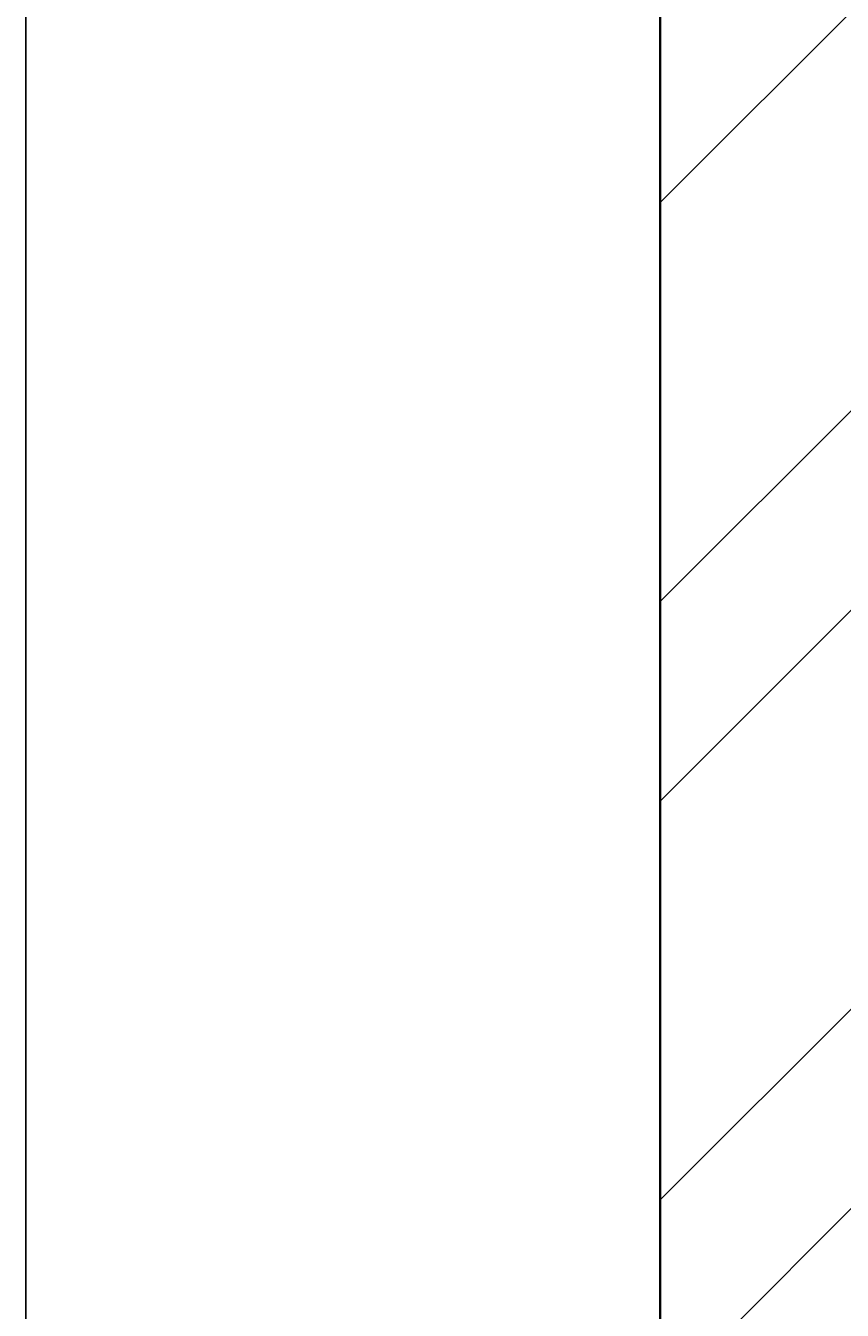
# Model space of a CAD drawing. Units: inches. Extents: x 1962 to 2771, y 1245 to 2660.
# Tile 48 of 114: x 2072 to 2090, y 2151 to 2180. Entities that reach past the tile are written whole.
import ezdxf

# ---------------------------------------------------------------- set-up
doc = ezdxf.new("R2010")
doc.units = ezdxf.units.IN
for name, color, linetype, lineweight in [('A-ANNO-DIMS', 2, 'Continuous', 18), ('A-WALL', 7, 'Continuous', 35), ('A-WALL-PATT', 252, 'Continuous', 13)]:
    doc.layers.add(name, color=color, linetype=linetype, lineweight=lineweight)
doc.styles.get("Standard").update_dxf_attribs({"font": 'arial.ttf'})
doc.dimstyles.get("Standard").update_dxf_attribs({"dimtxt": 0.18, "dimasz": 0.18, "dimexe": 0.18, "dimexo": 0.0625, "dimgap": 0.09, "dimtad": 0, "dimtih": 1, "dimtoh": 1, "dimdec": 4, "dimzin": 0, "dimdsep": 46, "dimtxsty": 'Standard', "dimcen": 0.09, "dimadec": 0, "dimazin": 0, "dimtfac": 1, "dimtdec": 4, "dimtofl": 0, "dimtmove": 0, "dimatfit": 3, "dimfxl": 1, "dimtolj": 1, "dimtzin": 0, "dimarcsym": 0})

# ---------------------------------------------------------------- blocks, each defined once
blk = doc.blocks.new('*D40')
at = {"layer": 'A-ANNO-DIMS', "color": 0, "lineweight": -2, "transparency": 16777216}
for p, q in [((2072.02, 2033.906), (2072.02, 2583.474)), ((2072.2, 2583.294), (2366.02, 2583.294)), ((2660.627, 2583.294), (2366.808, 2583.294)), ((2660.807, 2524.406), (2660.807, 2583.474))]:
    blk.add_line(p, q, dxfattribs=at)
at = {"layer": 'A-ANNO-DIMS', "color": 0, "transparency": 16777216}
for points in [[(2072.2, 2583.324), (2072.2, 2583.264), (2072.02, 2583.294)], [(2660.627, 2583.324), (2660.627, 2583.264), (2660.807, 2583.294)]]:
    blk.add_solid(points, dxfattribs=at)
at = {"layer": 'Defpoints', "color": 0, "transparency": 16777216}
for p in [(2660.807, 2583.294), (2660.807, 2524.344), (2072.02, 2033.844)]:
    blk.add_point(p, dxfattribs=at)
at = {"layer": 'A-ANNO-DIMS', "color": 0, "transparency": 16777216, "insert": (2366.414, 2583.294), "char_height": 0.18, "attachment_point": 5}
blk.add_mtext('\\A1;588.8', dxfattribs=at)
blk = doc.blocks.new('*D43')
at = {"layer": 'A-ANNO-DIMS', "color": 0, "lineweight": -2, "transparency": 16777216}
for p, q in [((2086.245, 2524.344), (2012.89, 2524.344)), ((2013.07, 2524.164), (2013.07, 2279.276)), ((2013.07, 2034.024), (2013.07, 2278.912)), ((2071.958, 2033.844), (2012.89, 2033.844))]:
    blk.add_line(p, q, dxfattribs=at)
at = {"layer": 'A-ANNO-DIMS', "color": 0, "transparency": 16777216}
for points in [[(2013.04, 2524.164), (2013.1, 2524.164), (2013.07, 2524.344)], [(2013.04, 2034.024), (2013.1, 2034.024), (2013.07, 2033.844)]]:
    blk.add_solid(points, dxfattribs=at)
at = {"layer": 'Defpoints', "color": 0, "transparency": 16777216}
for p in [(2086.307, 2524.344), (2013.07, 2033.844), (2072.02, 2033.844)]:
    blk.add_point(p, dxfattribs=at)
at = {"layer": 'A-ANNO-DIMS', "color": 0, "transparency": 16777216, "insert": (2013.07, 2279.094), "char_height": 0.18, "attachment_point": 5}
blk.add_mtext('\\A1;490.5', dxfattribs=at)

msp = doc.modelspace()

# ---------------------------------------------------------------- hatches: boundary and pattern name
at = {"layer": 'A-WALL-PATT'}
h = msp.add_hatch(dxfattribs=at)
h.set_pattern_fill('ANSI32', color=256)
h.paths.add_polyline_path([(2090.8074, 2467.3437), (2141.6481, 2467.3437), (2141.6481, 2469.5937), (2141.6481, 2471.8437), (2086.3074, 2471.8437), (2086.3074, 2422.5333), (2090.8074, 2422.5333)])
h.paths.add_polyline_path([(2282.7664, 2471.8437), (2204.8982, 2471.8437), (2204.8982, 2467.3437), (2234.8074, 2467.3437), (2234.8074, 2311.3437), (2228.7492, 2311.3437), (2228.7492, 2306.8437), (2234.8074, 2306.8437), (2331.9227, 2306.8437), (2331.9227, 2309.0937), (2331.9227, 2311.3437), (2239.3074, 2311.3437), (2239.3074, 2467.3437), (2282.7664, 2467.3437), (2282.7664, 2469.5937)])
h.paths.add_polyline_path([(2471.4531, 2519.8437), (2552.011, 2519.8437), (2564.3996, 2519.8437), (2564.3996, 2511.1389), (2568.8996, 2511.1389), (2568.8996, 2524.3437), (2466.9531, 2524.3437), (2466.9531, 2471.8437), (2450.0749, 2471.8437), (2446.4672, 2471.8437), (2446.4672, 2467.3437), (2450.0749, 2467.3437), (2475.9988, 2467.3437), (2475.9988, 2469.5937), (2475.9988, 2471.8437), (2471.4531, 2471.8437)])
h.paths.add_polyline_path([(2575.2231, 2469.5937), (2575.2231, 2471.8437), (2568.8996, 2471.8437), (2568.8996, 2487.1389), (2564.3996, 2487.1389), (2564.3996, 2471.8437), (2556.511, 2471.8437), (2499.2904, 2471.8437), (2499.2904, 2467.3437), (2507.8074, 2467.3437), (2507.8074, 2311.3437), (2414.863, 2311.3437), (2414.863, 2306.8437), (2512.3074, 2306.8437), (2517.0114, 2306.8437), (2517.0114, 2309.0937), (2517.0114, 2311.3437), (2512.3074, 2311.3437), (2512.3074, 2467.3437), (2575.2231, 2467.3437)])
h.paths.add_polyline_path([(2660.8074, 2471.8437), (2600.9602, 2471.8437), (2600.9602, 2467.3437), (2656.3074, 2467.3437), (2656.3074, 2432.5704), (2660.8074, 2432.5704)])
h.paths.add_polyline_path([(2660.8074, 2372.5704), (2656.3074, 2372.5704), (2656.3074, 2311.3437), (2600.276, 2311.3437), (2600.276, 2309.0937), (2600.276, 2306.8437), (2656.3074, 2306.8437), (2656.3074, 2296.2593), (2660.8074, 2296.2593)])
h.paths.add_polyline_path([(2572.3074, 2306.8437), (2577.1385, 2306.8437), (2577.1385, 2311.3437), (2551.082, 2311.3437), (2551.082, 2306.8437), (2567.8074, 2306.8437), (2567.8074, 2258.8437), (2540.0574, 2258.8437), (2540.0574, 2256.5937), (2540.0574, 2254.3437), (2567.8074, 2254.3437), (2656.3074, 2254.3437), (2656.3074, 2236.9085), (2660.8074, 2236.9085), (2660.8074, 2272.2593), (2656.3074, 2272.2593), (2656.3074, 2258.8437), (2572.3074, 2258.8437)])
h.paths.add_polyline_path([(2512.3074, 2254.3437), (2518.8716, 2254.3437), (2518.8716, 2256.5937), (2518.8716, 2258.8437), (2507.8074, 2258.8437), (2507.8074, 2177.8437), (2567.8074, 2177.8437), (2567.8074, 2172.9628), (2572.3074, 2172.9628), (2572.3074, 2177.8437), (2656.3074, 2177.8437), (2656.3074, 2166.4846), (2660.8074, 2166.4846), (2660.8074, 2200.9085), (2656.3074, 2200.9085), (2656.3074, 2182.3437), (2512.3074, 2182.3437)])
h.paths.add_polyline_path([(2656.3074, 2129.8437), (2572.3074, 2129.8437), (2572.3074, 2150.3044), (2570.0574, 2150.3044), (2567.8074, 2150.3044), (2567.8074, 2129.8437), (2507.8074, 2129.8437), (2507.8074, 2116.3027), (2510.0574, 2116.3027), (2512.3074, 2116.3027), (2512.3074, 2125.3437), (2567.8074, 2125.3437), (2572.3074, 2125.3437), (2656.3074, 2125.3437)])
h.paths.add_polyline_path([(2090.8074, 2362.5333), (2086.3074, 2362.5333), (2086.3074, 2298.6242), (2090.8074, 2298.6242), (2090.8074, 2306.8437), (2174.8074, 2306.8437), (2174.8074, 2286.4178), (2179.3074, 2286.4178), (2179.3074, 2306.8437), (2192.8641, 2306.8437), (2192.8641, 2309.0937), (2192.8641, 2311.3437), (2090.8074, 2311.3437)])
h.paths.add_polyline_path([(2209.156, 2258.8437), (2179.3074, 2258.8437), (2179.3074, 2263.2236), (2177.0574, 2263.2236), (2174.8074, 2263.2236), (2174.8074, 2258.8437), (2090.8074, 2258.8437), (2090.8074, 2274.6242), (2086.3074, 2274.6242), (2086.3074, 2238.2967), (2088.5574, 2238.2967), (2090.8074, 2238.2967), (2090.8074, 2254.3437), (2209.156, 2254.3437)])
h.paths.add_polyline_path([(2090.8074, 2177.8437), (2234.8074, 2177.8437), (2234.8074, 2173.1428), (2239.3074, 2173.1428), (2239.3074, 2258.8437), (2230.8442, 2258.8437), (2230.8442, 2256.5937), (2230.8442, 2254.3437), (2234.8074, 2254.3437), (2234.8074, 2182.3437), (2090.8074, 2182.3437), (2090.8074, 2202.2967), (2086.3074, 2202.2967), (2086.3074, 2140.0389), (2090.8074, 2140.0389)])
h.paths.add_polyline_path([(2090.8074, 2080.0389), (2086.3074, 2080.0389), (2086.3074, 2033.8437), (2090.8074, 2033.8437)], flags=17)
h.paths.add_polyline_path([(2244.9405, 2033.8437), (2239.3074, 2033.8437), (2239.3074, 2142.0665), (2237.2592, 2142.0665), (2234.8074, 2142.0665), (2234.8074, 2033.8437), (2090.8074, 2033.8437), (2076.5204, 2033.8437), (2072.0204, 2033.8437), (2072.0204, 2000.4493), (2076.5204, 2000.4493), (2076.5204, 2029.3437), (2090.8074, 2029.3437), (2244.9405, 2029.3437), (2244.9405, 2031.5937)])
h.paths.add_polyline_path([(2234.8074, 1933.3437), (2076.5204, 1933.3437), (2076.5204, 1952.4493), (2074.2704, 1952.4493), (2072.0204, 1952.4493), (2072.0204, 1933.3437), (2072.0204, 1928.8437), (2234.8074, 1928.8437)])
h.paths.add_polyline_path([(2090.8074, 1928.8437), (2086.3074, 1928.8437), (2086.3074, 1906.5013), (2090.8074, 1906.5013)])
h.paths.add_polyline_path([(2090.8074, 1846.5013), (2086.3074, 1846.5013), (2086.3074, 1769.9917), (2088.5574, 1769.9917), (2090.8074, 1769.9917), (2090.8074, 1780.3437), (2234.8074, 1780.3437), (2234.8074, 1708.3437), (2230.3764, 1708.3437), (2230.3764, 1703.8437), (2239.3074, 1703.8437), (2239.3074, 1792.6669), (2237.0574, 1792.6669), (2234.8074, 1792.6669), (2234.8074, 1784.8437), (2090.8074, 1784.8437)])
h.paths.add_polyline_path([(2239.3074, 1928.8437), (2244.9405, 1928.8437), (2244.9405, 1931.0937), (2244.9405, 1933.3437), (2234.8074, 1933.3437), (2234.8074, 1928.8437), (2234.8074, 1825.5949), (2239.3074, 1825.5949)])
h.paths.add_polyline_path([(2148.0425, 1649.0937), (2148.0425, 1651.3437), (2090.8074, 1651.3437), (2090.8074, 1646.8437), (2148.0425, 1646.8437)], flags=0)
h.paths.add_polyline_path([(2207.5601, 1708.3437), (2090.8074, 1708.3437), (2090.8074, 1703.8437), (2174.8074, 1703.8437), (2174.8074, 1651.3437), (2170.4457, 1651.3437), (2170.4457, 1646.8437), (2195.9924, 1646.8437), (2195.9924, 1649.0937), (2195.9924, 1651.3437), (2179.3074, 1651.3437), (2179.3074, 1703.8437), (2207.5601, 1703.8437), (2207.5601, 1706.0937)])
h.paths.add_polyline_path([(2090.8074, 1733.9917), (2086.3074, 1733.9917), (2086.3074, 1696.1032), (2088.5574, 1696.1032), (2090.8074, 1696.1032)])
h.paths.add_polyline_path([(2090.8074, 1672.1032), (2086.3074, 1672.1032), (2086.3074, 1600.3335), (2090.8074, 1600.3335)])
h.paths.add_polyline_path([(2090.8074, 1540.3335), (2086.3074, 1540.3335), (2086.3074, 1486.3437), (2139.6766, 1486.3437), (2139.6766, 1490.8437), (2090.8074, 1490.8437)])
h.paths.add_polyline_path([(2302.3876, 1490.8437), (2239.3074, 1490.8437), (2239.3074, 1646.8437), (2335.9994, 1646.8437), (2335.9994, 1651.3437), (2229.884, 1651.3437), (2229.884, 1646.8437), (2234.8074, 1646.8437), (2234.8074, 1490.8437), (2202.7103, 1490.8437), (2202.7103, 1488.5937), (2202.7103, 1486.3437), (2275.0699, 1486.3437), (2275.0699, 1475.772), (2279.5699, 1475.772), (2279.5699, 1486.3437), (2302.3876, 1486.3437)])
h.paths.add_polyline_path([(2279.5699, 1451.772), (2275.0699, 1451.772), (2275.0699, 1438.3437), (2174.8074, 1438.3437), (2174.8074, 1486.3437), (2179.7922, 1486.3437), (2179.7922, 1490.8437), (2163.3585, 1490.8437), (2163.3585, 1488.5937), (2163.3585, 1486.3437), (2170.3074, 1486.3437), (2170.3074, 1433.8437), (2279.5699, 1433.8437)])
h.paths.add_polyline_path([(2427.2363, 1490.8437), (2375.8074, 1490.8437), (2375.8074, 1646.8437), (2381.6401, 1646.8437), (2381.6401, 1651.3437), (2365.887, 1651.3437), (2365.887, 1649.0937), (2365.887, 1646.8437), (2371.3074, 1646.8437), (2371.3074, 1490.8437), (2327.5627, 1490.8437), (2327.5627, 1488.5937), (2327.5627, 1486.3437), (2371.3074, 1486.3437), (2371.3074, 1433.8437), (2375.8074, 1433.8437), (2375.8074, 1486.3437), (2427.2363, 1486.3437)])
h.paths.add_polyline_path([(2512.3074, 1646.8437), (2519.4351, 1646.8437), (2519.4351, 1649.0937), (2519.4351, 1651.3437), (2507.8074, 1651.3437), (2416.0063, 1651.3437), (2416.0063, 1649.0937), (2416.0063, 1646.8437), (2507.8074, 1646.8437), (2507.8074, 1490.8437), (2497.0532, 1490.8437), (2497.0532, 1488.5937), (2497.0532, 1486.3437), (2574.9344, 1486.3437), (2574.9344, 1476.0181), (2579.4344, 1476.0181), (2579.4344, 1486.3437), (2584.4872, 1486.3437), (2584.3074, 1490.8437), (2512.3074, 1490.8437)])
h.paths.add_polyline_path([(2470.5091, 1486.3437), (2473.9767, 1486.3437), (2473.9767, 1490.8437), (2449.6605, 1490.8437), (2449.6605, 1488.5937), (2449.6605, 1486.3437), (2466.0091, 1486.3437), (2466.0091, 1433.8437), (2470.5091, 1433.8437), (2579.4344, 1433.8437), (2579.4344, 1452.0181), (2574.9344, 1452.0181), (2574.9344, 1438.3437), (2554.5091, 1438.3437), (2470.5091, 1438.3437)])
h.paths.add_polyline_path([(2656.3074, 1490.8437), (2611.86, 1490.8437), (2611.86, 1486.3437), (2656.3074, 1486.3437)])
h.paths.add_polyline_path([(2660.8074, 1532.7007), (2658.5574, 1532.7007), (2656.3074, 1532.7007), (2656.3074, 1486.3437), (2660.8074, 1486.3437)])
h.paths.add_polyline_path([(2660.8074, 1664.9663), (2656.3074, 1664.9663), (2656.3074, 1651.3437), (2602.2313, 1651.3437), (2602.2313, 1646.8437), (2656.3074, 1646.8437), (2656.3074, 1592.7007), (2660.8074, 1592.7007)])
h.paths.add_polyline_path([(2660.8074, 1724.5221), (2656.3074, 1724.5221), (2656.3074, 1703.8437), (2542.4725, 1703.8437), (2542.4725, 1699.3437), (2567.8074, 1699.3437), (2567.8074, 1651.3437), (2552.7766, 1651.3437), (2552.7766, 1649.0937), (2552.7766, 1646.8437), (2577.2878, 1646.8437), (2577.2878, 1649.0937), (2577.2878, 1651.3437), (2572.3074, 1651.3437), (2572.3074, 1699.3437), (2656.3074, 1699.3437), (2656.3074, 1688.9663), (2660.8074, 1688.9663)])
h.paths.add_polyline_path([(2660.8074, 1880.6524), (2656.3074, 1880.6524), (2656.3074, 1832.8437), (2512.3074, 1832.8437), (2512.3074, 1837.8959), (2507.8074, 1837.8959), (2507.8074, 1828.3437), (2567.8074, 1828.3437), (2567.8074, 1804.3437), (2572.3074, 1804.3437), (2572.3074, 1828.3437), (2656.3074, 1828.3437), (2656.3074, 1818.6778), (2660.8074, 1818.6778)])
h.paths.add_polyline_path([(2660.8074, 1794.6778), (2656.3074, 1794.6778), (2656.3074, 1780.3437), (2572.3074, 1780.3437), (2572.3074, 1783.0303), (2570.0574, 1783.0303), (2567.8074, 1783.0303), (2567.8074, 1780.3437), (2507.8074, 1780.3437), (2507.8074, 1699.3437), (2517.8858, 1699.3437), (2517.8858, 1701.5937), (2517.8858, 1703.8437), (2512.3074, 1703.8437), (2512.3074, 1775.8437), (2656.3074, 1775.8437), (2656.3074, 1760.5221), (2660.8074, 1760.5221)])
h.paths.add_polyline_path([(2660.8074, 1981.3437), (2660.8074, 2020.2808), (2658.5574, 2020.2808), (2656.3074, 2020.2808), (2656.3074, 1981.3437), (2512.3074, 1981.3437), (2512.3074, 2086.6996), (2507.8074, 2086.6996), (2507.8074, 1981.3437), (2375.8074, 1981.3437), (2375.8074, 1986.8505), (2373.5574, 1986.8505), (2371.3074, 1986.8505), (2371.3074, 1973.2607), (2375.8074, 1973.2607), (2375.8074, 1976.8437), (2507.8074, 1976.8437), (2507.8074, 1865.4281), (2510.0574, 1865.4281), (2512.3074, 1865.4281), (2512.3074, 1976.8437), (2660.8074, 1976.8437)])
h.paths.add_polyline_path([(2375.8074, 1940.297), (2373.5574, 1940.297), (2371.3074, 1940.297), (2371.3074, 1933.3437), (2278.4434, 1933.3437), (2278.4434, 1928.8437), (2371.3074, 1928.8437), (2371.3074, 1651.3437), (2375.8074, 1651.3437)])
h.paths.add_polyline_path([(2660.8074, 1976.8437), (2656.3074, 1976.8437), (2656.3074, 1940.6524), (2660.8074, 1940.6524)], flags=17)
h.paths.add_polyline_path([(2660.8074, 2142.4846), (2656.3074, 2142.4846), (2656.3074, 2080.2808), (2660.8074, 2080.2808)])
h.paths.add_polyline_path([(2381.4189, 2311.3437), (2375.8074, 2311.3437), (2375.8074, 2467.3437), (2424.7242, 2467.3437), (2424.7242, 2469.5937), (2424.7242, 2471.8437), (2375.8074, 2471.8437), (2375.8074, 2524.3437), (2371.3074, 2524.3437), (2371.3074, 2471.8437), (2307.2097, 2471.8437), (2307.2097, 2467.3437), (2371.3074, 2467.3437), (2371.3074, 2311.3437), (2366.8901, 2311.3437), (2366.8901, 2306.8437), (2371.3074, 2306.8437), (2371.3074, 2033.8437), (2279.6589, 2033.8437), (2279.6589, 2029.3437), (2371.3074, 2029.3437), (2371.3074, 2014.2598), (2375.8074, 2014.2598), (2375.8074, 2306.8437), (2381.4189, 2306.8437)])
h.paths.add_polyline_path([(2263.3074, 2524.3437), (2170.3074, 2524.3437), (2170.3074, 2519.8437), (2170.3074, 2471.8437), (2165.0312, 2471.8437), (2165.0312, 2467.3437), (2179.6721, 2467.3437), (2179.6721, 2469.5161), (2179.6721, 2471.8437), (2174.8074, 2471.8437), (2174.8074, 2519.8437), (2258.8074, 2519.8437), (2258.8074, 2511.6436), (2263.3074, 2511.6436)])
h.paths.add_polyline_path([(2245.0232, 1361.4123), (2492.9468, 1361.4123), (2492.9468, 1398.505), (2245.0232, 1398.505)], flags=9)
h.paths.add_polyline_path([(2388.1434, 2086.6936), (2425.0704, 2086.6936), (2425.0704, 2105.3509), (2388.1434, 2105.3509)], flags=9)
h.paths.add_polyline_path([(2404.922, 2242.6744), (2445.7337, 2242.6744), (2445.7337, 2261.3318), (2404.922, 2261.3318)], flags=9)
h.paths.add_polyline_path([(2269.4107, 2156.7935), (2306.3378, 2156.7935), (2306.3378, 2175.4508), (2269.4107, 2175.4508)], flags=9)
h.paths.add_polyline_path([(2269.3277, 2233.4343), (2306.2547, 2233.4343), (2306.2547, 2252.0917), (2269.3277, 2252.0917)], flags=9)
h.paths.add_polyline_path([(2431.6052, 2320.6922), (2470.4456, 2320.6922), (2470.4456, 2339.3495), (2431.6052, 2339.3495)], flags=25)
h.paths.add_polyline_path([(2249.6902, 2315.7608), (2288.5306, 2315.7608), (2288.5306, 2334.4182), (2249.6902, 2334.4182)], flags=25)
h.paths.add_polyline_path([(2096.9301, 2314.3181), (2135.7704, 2314.3181), (2135.7704, 2332.9755), (2096.9301, 2332.9755)], flags=25)
h.paths.add_polyline_path([(2134.3475, 2285.7089), (2161.4655, 2285.7089), (2161.4655, 2304.3662), (2134.3475, 2304.3662)], flags=9)
h.paths.add_polyline_path([(2126.5155, 2209.4076), (2159.9227, 2209.4076), (2159.9227, 2228.065), (2126.5155, 2228.065)], flags=25)
h.paths.add_polyline_path([(2110.5753, 2141.5299), (2149.4157, 2141.5299), (2149.4157, 2160.1872), (2110.5753, 2160.1872)], flags=25)
h.paths.add_polyline_path([(2249.8618, 1968.3317), (2286.3966, 1968.3317), (2286.3966, 1986.989), (2249.8618, 1986.989)], flags=9)
h.paths.add_polyline_path([(2395.9507, 1777.0051), (2436.7624, 1777.0051), (2436.7624, 1795.6625), (2395.9507, 1795.6625)], flags=9)
h.paths.add_polyline_path([(2398.5259, 1888.5651), (2435.0062, 1888.5651), (2435.0062, 1907.2224), (2398.5259, 1907.2224)], flags=25)
h.paths.add_polyline_path([(2259.3506, 1728.3559), (2296.2776, 1728.3559), (2296.2776, 1747.0132), (2259.3506, 1747.0132)], flags=9)
h.paths.add_polyline_path([(2271.3698, 1845.268), (2308.2968, 1845.268), (2308.2968, 1863.9253), (2271.3698, 1863.9253)], flags=9)
h.paths.add_polyline_path([(2120.9355, 1786.3027), (2159.7759, 1786.3027), (2159.7759, 1804.9601), (2120.9355, 1804.9601)], flags=25)
h.paths.add_polyline_path([(2121.3164, 1732.1043), (2154.7236, 1732.1043), (2154.7236, 1750.7616), (2121.3164, 1750.7616)], flags=25)
h.paths.add_polyline_path([(2118.3706, 1678.8997), (2147.5282, 1678.8997), (2147.5282, 1697.557), (2118.3706, 1697.557)], flags=25)
h.paths.add_polyline_path([(2385.9227, 1493.557), (2424.763, 1493.557), (2424.763, 1512.2143), (2385.9227, 1512.2143)], flags=25)
h.paths.add_polyline_path([(2248.7058, 1500.0256), (2287.5462, 1500.0256), (2287.5462, 1518.6829), (2248.7058, 1518.6829)], flags=25)
h.paths.add_polyline_path([(2104.1669, 1617.3771), (2143.0073, 1617.3771), (2143.0073, 1636.0344), (2104.1669, 1636.0344)], flags=9)
h.paths.add_polyline_path([(2096.0714, 1447.8824), (2137.3845, 1447.8824), (2137.3845, 1458.1859), (2096.0714, 1458.1859)], flags=9)
h.paths.add_polyline_path([(2180.6114, 1440.325), (2209.7689, 1440.325), (2209.7689, 1458.9823), (2180.6114, 1458.9823)], flags=25)
h.paths.add_polyline_path([(2316.1698, 1447.9637), (2357.4829, 1447.9637), (2357.4829, 1458.2673), (2316.1698, 1458.2673)], flags=9)
h.paths.add_polyline_path([(2397.6187, 1447.9637), (2438.9318, 1447.9637), (2438.9318, 1458.2673), (2397.6187, 1458.2673)], flags=9)
h.paths.add_polyline_path([(2473.0778, 1439.5953), (2502.2354, 1439.5953), (2502.2354, 1458.2527), (2473.0778, 1458.2527)], flags=25)
h.paths.add_polyline_path([(2589.7027, 1447.8819), (2631.0158, 1447.8819), (2631.0158, 1458.1855), (2589.7027, 1458.1855)], flags=9)
h.paths.add_polyline_path([(2522.4009, 1497.5285), (2561.2413, 1497.5285), (2561.2413, 1516.1859), (2522.4009, 1516.1859)], flags=25)
h.paths.add_polyline_path([(2579.6565, 1671.3482), (2608.8141, 1671.3482), (2608.8141, 1690.0056), (2579.6565, 1690.0056)], flags=25)
h.paths.add_polyline_path([(2544.7038, 1725.5064), (2578.1111, 1725.5064), (2578.1111, 1744.1637), (2544.7038, 1744.1637)], flags=25)
h.paths.add_polyline_path([(2578.1191, 1807.472), (2607.2766, 1807.472), (2607.2766, 1826.1293), (2578.1191, 1826.1293)], flags=25)
h.paths.add_polyline_path([(2595.0614, 1835.1839), (2633.9018, 1835.1839), (2633.9018, 1853.8413), (2595.0614, 1853.8413)], flags=25)
h.paths.add_polyline_path([(2567.0097, 2097.7035), (2605.8501, 2097.7035), (2605.8501, 2116.3609), (2567.0097, 2116.3609)], flags=9)
h.paths.add_polyline_path([(2586.644, 2134.6454), (2615.8015, 2134.6454), (2615.8015, 2153.3027), (2586.644, 2153.3027)], flags=9)
h.paths.add_polyline_path([(2544.6185, 2212.6783), (2578.0258, 2212.6783), (2578.0258, 2231.3356), (2544.6185, 2231.3356)], flags=25)
h.paths.add_polyline_path([(2577.0273, 2256.9023), (2606.1849, 2256.9023), (2606.1849, 2275.5597), (2577.0273, 2275.5597)], flags=24)
h.paths.add_polyline_path([(2605.2683, 2315.2821), (2644.1087, 2315.2821), (2644.1087, 2333.9395), (2605.2683, 2333.9395)], flags=25)
h.paths.add_polyline_path([(2583.1244, 2496.1815), (2624.4375, 2496.1815), (2624.4375, 2506.4851), (2583.1244, 2506.4851)], flags=9)
h.paths.add_polyline_path([(2474.761, 2497.0823), (2503.9185, 2497.0823), (2503.9185, 2515.7397), (2474.761, 2515.7397)], flags=25)
h.paths.add_polyline_path([(2387.5787, 2494.2563), (2428.902, 2494.2563), (2428.902, 2504.5598), (2387.5787, 2504.5598)], flags=9)
h.paths.add_polyline_path([(2300.1657, 2500.1564), (2341.4788, 2500.1564), (2341.4788, 2510.46), (2300.1657, 2510.46)], flags=25)
h.paths.add_polyline_path([(2176.8589, 2497.5843), (2206.0165, 2497.5843), (2206.0165, 2516.2416), (2176.8589, 2516.2416)], flags=25)
h.paths.add_polyline_path([(2097.4668, 2494.9762), (2138.7799, 2494.9762), (2138.7799, 2505.2798), (2097.4668, 2505.2798)], flags=9)

# ---------------------------------------------------------------- linework, layer by layer
at = {"layer": 'A-WALL'}
msp.add_line((2086.3074, 2471.8437), (2086.3074, 2033.8437), dxfattribs=at)

# ---------------------------------------------------------------- dimensions: what is measured, and where the dimension line sits
at = {"layer": 'A-ANNO-DIMS'}
dim = msp.add_linear_dim(base=(2660.8074, 2583.2937), p1=(2072.0204, 2033.8437), p2=(2660.8074, 2524.3437), dimstyle='Standard', override={"dimdec": 1, "dimlfac": 1, "dimrnd": 0, "dimzin": 0, "dimdsep": 46, "dimlunit": 2}, dxfattribs=at)
dim.commit()
dim.dimension.update_dxf_attribs({"geometry": '*D40', "text_midpoint": (2366.4139, 2583.2937)})
dim = msp.add_linear_dim(base=(2013.0704, 2033.8437), p1=(2086.3074, 2524.3437), p2=(2072.0204, 2033.8437), angle=90, dimstyle='Standard', override={"dimdec": 1, "dimlfac": 1, "dimrnd": 0, "dimzin": 0, "dimdsep": 46, "dimlunit": 2}, dxfattribs=at)
dim.commit()
dim.dimension.update_dxf_attribs({"geometry": '*D43', "text_midpoint": (2013.0704, 2279.0937)})

doc.saveas('drawing.dxf')
